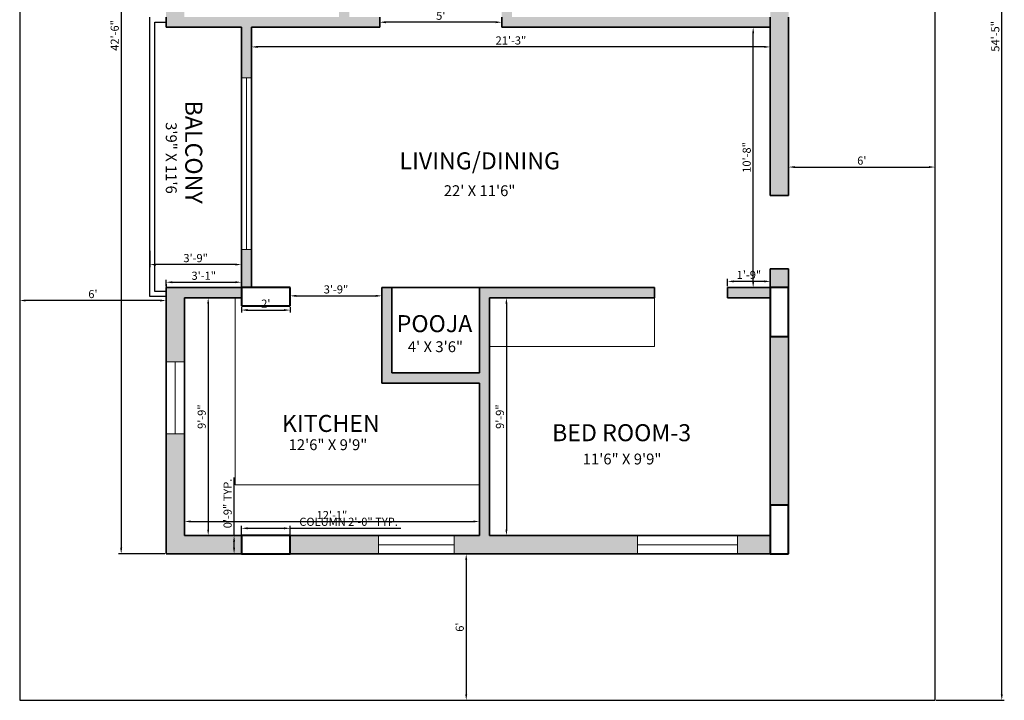
# Model space of a CAD drawing. Units: millimetres. Extents: x 2190 to 2674, y 1487 to 2179.
# Tile 1 of 2: x 2190 to 2674, y 1487 to 1822. Entities that reach past the tile are written whole.
import ezdxf

# ---------------------------------------------------------------- set-up
doc = ezdxf.new("R2010")
doc.units = ezdxf.units.MM
for name, color, linetype, lineweight in [('A-ANNO-DIMS', 2, 'Continuous', 18), ('A-AREA-IDEN', 7, 'Continuous', 18), ('A-WALL', 7, 'Continuous', 35), ('C-PROP', 7, 'Continuous', 25)]:
    doc.layers.add(name, color=color, linetype=linetype, lineweight=lineweight)
for name, color, linetype, lineweight, true_color in [('A-COLS', 240, 'Continuous', 40, 0xed1f24), ('A-FLOR-CASE', 177, 'Continuous', 18, 0x293189), ('A-FLOR-HRAL', 177, 'Continuous', 25, 0x293189), ('A-GLAZ', 177, 'Continuous', 18, 0x293189), ('A-WALL-PATT', 32, 'Continuous', 13, 0xcd6928)]:
    doc.layers.add(name, color=color, linetype=linetype, lineweight=lineweight, true_color=true_color)
doc.styles.get("Standard").update_dxf_attribs({"font": 'arial.ttf'})
doc.dimstyles.new('ISO-25', dxfattribs={"dimtxt": 4, "dimasz": 3, "dimexe": 1.25, "dimexo": 0.625, "dimtad": 1, "dimdec": 0, "dimlunit": 3, "dimtxsty": 'Standard', "dimcen": 2.5, "dimadec": 0, "dimazin": 0, "dimtfac": 1, "dimtdec": 0, "dimtmove": 0, "dimatfit": 3, "dimfxl": 1, "dimarcsym": 0})

# ---------------------------------------------------------------- blocks, each defined once
blk = doc.blocks.new('*D4')
at = {"layer": 'A-ANNO-DIMS', "color": 0, "lineweight": -2, "transparency": 16777216}
for p, q in [((2254.11, 1708.51), (2254.11, 1700.51)), ((2299.11, 1708.51), (2299.11, 1700.51)), ((2296.11, 1701.76), (2257.11, 1701.76))]:
    blk.add_line(p, q, dxfattribs=at)
at = {"layer": 'A-ANNO-DIMS', "color": 0, "transparency": 16777216}
for points in [[(2257.11, 1702.26), (2257.11, 1701.26), (2254.11, 1701.76)], [(2296.11, 1702.26), (2296.11, 1701.26), (2299.11, 1701.76)]]:
    blk.add_solid(points, dxfattribs=at)
at = {"layer": 'Defpoints', "color": 0, "transparency": 16777216}
for p in [(2254.11, 1709.13), (2299.11, 1709.13), (2254.11, 1701.76)]:
    blk.add_point(p, dxfattribs=at)
at = {"layer": 'A-ANNO-DIMS', "color": 0, "transparency": 16777216, "insert": (2276.61, 1704.43), "char_height": 4, "attachment_point": 5}
blk.add_mtext('3\'-9"', dxfattribs=at)
blk = doc.blocks.new('*D5')
at = {"layer": 'A-ANNO-DIMS', "color": 0, "lineweight": -2, "transparency": 16777216}
for p, q in [((2262.11, 1691.07), (2262.11, 1694.32)), ((2299.11, 1691.07), (2299.11, 1694.32)), ((2265.11, 1693.07), (2296.11, 1693.07))]:
    blk.add_line(p, q, dxfattribs=at)
at = {"layer": 'A-ANNO-DIMS', "color": 0, "transparency": 16777216}
for points in [[(2265.11, 1693.57), (2265.11, 1692.57), (2262.11, 1693.07)], [(2296.11, 1693.57), (2296.11, 1692.57), (2299.11, 1693.07)]]:
    blk.add_solid(points, dxfattribs=at)
at = {"layer": 'Defpoints', "color": 0, "transparency": 16777216}
for p in [(2262.11, 1690.45), (2299.11, 1693.07), (2299.11, 1690.45)]:
    blk.add_point(p, dxfattribs=at)
at = {"layer": 'A-ANNO-DIMS', "color": 0, "transparency": 16777216, "insert": (2280.61, 1695.74), "char_height": 4, "attachment_point": 5}
blk.add_mtext('3\'-1"', dxfattribs=at)
blk = doc.blocks.new('*D6')
at = {"layer": 'A-ANNO-DIMS', "color": 0, "lineweight": -2, "transparency": 16777216}
for p, q in [((2299.11, 1680.82), (2299.11, 1678.13)), ((2323.11, 1680.82), (2323.11, 1678.13)), ((2302.11, 1679.38), (2320.11, 1679.38))]:
    blk.add_line(p, q, dxfattribs=at)
at = {"layer": 'A-ANNO-DIMS', "color": 0, "transparency": 16777216}
for points in [[(2302.11, 1679.88), (2302.11, 1678.88), (2299.11, 1679.38)], [(2320.11, 1679.88), (2320.11, 1678.88), (2323.11, 1679.38)]]:
    blk.add_solid(points, dxfattribs=at)
at = {"layer": 'Defpoints', "color": 0, "transparency": 16777216}
for p in [(2299.11, 1681.45), (2323.11, 1681.45), (2323.11, 1679.38)]:
    blk.add_point(p, dxfattribs=at)
at = {"layer": 'A-ANNO-DIMS', "color": 0, "transparency": 16777216, "insert": (2311.11, 1682.02), "char_height": 4, "attachment_point": 5}
blk.add_mtext("2'", dxfattribs=at)
blk = doc.blocks.new('*D7')
at = {"layer": 'A-ANNO-DIMS', "color": 0, "lineweight": -2, "transparency": 16777216}
for p, q in [((2323.11, 1689.82), (2323.11, 1685.11)), ((2368.11, 1689.82), (2368.11, 1685.11)), ((2326.11, 1686.36), (2365.11, 1686.36))]:
    blk.add_line(p, q, dxfattribs=at)
at = {"layer": 'A-ANNO-DIMS', "color": 0, "transparency": 16777216}
for points in [[(2326.11, 1686.86), (2326.11, 1685.86), (2323.11, 1686.36)], [(2365.11, 1686.86), (2365.11, 1685.86), (2368.11, 1686.36)]]:
    blk.add_solid(points, dxfattribs=at)
at = {"layer": 'Defpoints', "color": 0, "transparency": 16777216}
for p in [(2323.11, 1690.45), (2368.11, 1690.45), (2368.11, 1686.36)]:
    blk.add_point(p, dxfattribs=at)
at = {"layer": 'A-ANNO-DIMS', "color": 0, "transparency": 16777216, "insert": (2345.61, 1689.03), "char_height": 4, "attachment_point": 5}
blk.add_mtext('3\'-9"', dxfattribs=at)
blk = doc.blocks.new('*D8')
at = {"layer": 'A-ANNO-DIMS', "color": 0, "lineweight": -2, "transparency": 16777216}
for p, q in [((2271.73, 1685.45), (2284.03, 1685.45)), ((2282.78, 1682.45), (2282.78, 1571.45)), ((2271.73, 1568.45), (2284.03, 1568.45))]:
    blk.add_line(p, q, dxfattribs=at)
at = {"layer": 'A-ANNO-DIMS', "color": 0, "transparency": 16777216}
for points in [[(2282.28, 1682.45), (2283.28, 1682.45), (2282.78, 1685.45)], [(2282.28, 1571.45), (2283.28, 1571.45), (2282.78, 1568.45)]]:
    blk.add_solid(points, dxfattribs=at)
at = {"layer": 'Defpoints', "color": 0, "transparency": 16777216}
for p in [(2271.11, 1685.45), (2271.11, 1568.45), (2282.78, 1568.45)]:
    blk.add_point(p, dxfattribs=at)
at = {"layer": 'A-ANNO-DIMS', "color": 0, "transparency": 16777216, "insert": (2280.11, 1626.95), "char_height": 4, "attachment_point": 5, "rotation": 90}
blk.add_mtext('9\'-9"', dxfattribs=at)
blk = doc.blocks.new('*D9')
at = {"layer": 'A-ANNO-DIMS', "color": 0, "lineweight": -2, "transparency": 16777216}
for p, q in [((2271.11, 1569.07), (2271.11, 1576.65)), ((2274.11, 1575.4), (2413.11, 1575.4)), ((2416.11, 1569.07), (2416.11, 1576.65))]:
    blk.add_line(p, q, dxfattribs=at)
at = {"layer": 'A-ANNO-DIMS', "color": 0, "transparency": 16777216}
for points in [[(2274.11, 1575.9), (2274.11, 1574.9), (2271.11, 1575.4)], [(2413.11, 1575.9), (2413.11, 1574.9), (2416.11, 1575.4)]]:
    blk.add_solid(points, dxfattribs=at)
at = {"layer": 'Defpoints', "color": 0, "transparency": 16777216}
for p in [(2416.11, 1575.4), (2271.11, 1568.45), (2416.11, 1568.45)]:
    blk.add_point(p, dxfattribs=at)
at = {"layer": 'A-ANNO-DIMS', "color": 0, "transparency": 16777216, "insert": (2343.61, 1578.03), "char_height": 4, "attachment_point": 5}
blk.add_mtext('12\'-1"', dxfattribs=at)
blk = doc.blocks.new('*D10')
at = {"layer": 'A-ANNO-DIMS', "color": 0, "lineweight": -2, "transparency": 16777216}
for p, q in [((2421.73, 1685.45), (2430.64, 1685.45)), ((2429.39, 1682.45), (2429.39, 1571.45)), ((2421.73, 1568.45), (2430.64, 1568.45))]:
    blk.add_line(p, q, dxfattribs=at)
at = {"layer": 'A-ANNO-DIMS', "color": 0, "transparency": 16777216}
for points in [[(2428.89, 1682.45), (2429.89, 1682.45), (2429.39, 1685.45)], [(2428.89, 1571.45), (2429.89, 1571.45), (2429.39, 1568.45)]]:
    blk.add_solid(points, dxfattribs=at)
at = {"layer": 'Defpoints', "color": 0, "transparency": 16777216}
for p in [(2421.11, 1685.45), (2421.11, 1568.45), (2429.39, 1568.45)]:
    blk.add_point(p, dxfattribs=at)
at = {"layer": 'A-ANNO-DIMS', "color": 0, "transparency": 16777216, "insert": (2426.72, 1626.95), "char_height": 4, "attachment_point": 5, "rotation": 90}
blk.add_mtext('9\'-9"', dxfattribs=at)
blk = doc.blocks.new('*D11')
at = {"layer": 'A-ANNO-DIMS', "color": 0, "lineweight": -2, "transparency": 16777216}
for p, q in [((2538.11, 1691.07), (2538.11, 1694.73)), ((2559.11, 1691.07), (2559.11, 1694.73)), ((2556.11, 1693.48), (2541.11, 1693.48))]:
    blk.add_line(p, q, dxfattribs=at)
at = {"layer": 'A-ANNO-DIMS', "color": 0, "transparency": 16777216}
for points in [[(2541.11, 1693.98), (2541.11, 1692.98), (2538.11, 1693.48)], [(2556.11, 1693.98), (2556.11, 1692.98), (2559.11, 1693.48)]]:
    blk.add_solid(points, dxfattribs=at)
at = {"layer": 'Defpoints', "color": 0, "transparency": 16777216}
for p in [(2538.11, 1693.48), (2538.11, 1690.45), (2559.11, 1690.45)]:
    blk.add_point(p, dxfattribs=at)
at = {"layer": 'A-ANNO-DIMS', "color": 0, "transparency": 16777216, "insert": (2548.61, 1696.15), "char_height": 4, "attachment_point": 5}
blk.add_mtext('1\'-9"', dxfattribs=at)
blk = doc.blocks.new('*D12')
at = {"layer": 'A-ANNO-DIMS', "color": 0, "lineweight": -2, "transparency": 16777216}
for p, q in [((2558.48, 1818.45), (2549.45, 1818.45)), ((2550.7, 1693.45), (2550.7, 1815.45)), ((2558.48, 1690.45), (2549.45, 1690.45))]:
    blk.add_line(p, q, dxfattribs=at)
at = {"layer": 'A-ANNO-DIMS', "color": 0, "transparency": 16777216}
for points in [[(2550.2, 1815.45), (2551.2, 1815.45), (2550.7, 1818.45)], [(2550.2, 1693.45), (2551.2, 1693.45), (2550.7, 1690.45)]]:
    blk.add_solid(points, dxfattribs=at)
at = {"layer": 'Defpoints', "color": 0, "transparency": 16777216}
for p in [(2550.7, 1818.45), (2559.11, 1818.45), (2559.11, 1690.45)]:
    blk.add_point(p, dxfattribs=at)
at = {"layer": 'A-ANNO-DIMS', "color": 0, "transparency": 16777216, "insert": (2548.03, 1754.45), "char_height": 4, "attachment_point": 5, "rotation": 90}
blk.add_mtext('10\'-8"', dxfattribs=at)
blk = doc.blocks.new('*D13')
at = {"layer": 'A-ANNO-DIMS', "color": 0, "lineweight": -2, "transparency": 16777216}
for p, q in [((2304.11, 1817.82), (2304.11, 1807.55)), ((2559.11, 1817.82), (2559.11, 1807.55)), ((2556.11, 1808.8), (2307.11, 1808.8))]:
    blk.add_line(p, q, dxfattribs=at)
at = {"layer": 'A-ANNO-DIMS', "color": 0, "transparency": 16777216}
for points in [[(2307.11, 1809.3), (2307.11, 1808.3), (2304.11, 1808.8)], [(2556.11, 1809.3), (2556.11, 1808.3), (2559.11, 1808.8)]]:
    blk.add_solid(points, dxfattribs=at)
at = {"layer": 'Defpoints', "color": 0, "transparency": 16777216}
for p in [(2304.11, 1818.45), (2559.11, 1818.45), (2304.11, 1808.8)]:
    blk.add_point(p, dxfattribs=at)
at = {"layer": 'A-ANNO-DIMS', "color": 0, "transparency": 16777216, "insert": (2431.61, 1811.47), "char_height": 4, "attachment_point": 5}
blk.add_mtext('21\'-3"', dxfattribs=at)
blk = doc.blocks.new('*D14')
at = {"layer": 'A-ANNO-DIMS', "color": 0, "lineweight": -2, "transparency": 16777216}
for p, q in [((2367.11, 1819.07), (2367.11, 1822.2)), ((2424.11, 1820.95), (2370.11, 1820.95)), ((2427.11, 1819.07), (2427.11, 1822.2))]:
    blk.add_line(p, q, dxfattribs=at)
at = {"layer": 'A-ANNO-DIMS', "color": 0, "transparency": 16777216}
for points in [[(2370.11, 1821.45), (2370.11, 1820.45), (2367.11, 1820.95)], [(2424.11, 1821.45), (2424.11, 1820.45), (2427.11, 1820.95)]]:
    blk.add_solid(points, dxfattribs=at)
at = {"layer": 'Defpoints', "color": 0, "transparency": 16777216}
for p in [(2367.11, 1820.95), (2367.11, 1818.45), (2427.11, 1818.45)]:
    blk.add_point(p, dxfattribs=at)
at = {"layer": 'A-ANNO-DIMS', "color": 0, "transparency": 16777216, "insert": (2397.11, 1823.61), "char_height": 4, "attachment_point": 5}
blk.add_mtext("5'", dxfattribs=at)
blk = doc.blocks.new('*D21')
at = {"layer": 'A-ANNO-DIMS', "color": 0, "lineweight": -2, "transparency": 16777216}
for p, q in [((2261.48, 2069.45), (2238.76, 2069.45)), ((2240.01, 2066.45), (2240.01, 1562.45)), ((2261.48, 1559.45), (2238.76, 1559.45))]:
    blk.add_line(p, q, dxfattribs=at)
at = {"layer": 'A-ANNO-DIMS', "color": 0, "transparency": 16777216}
for points in [[(2239.51, 2066.45), (2240.51, 2066.45), (2240.01, 2069.45)], [(2239.51, 1562.45), (2240.51, 1562.45), (2240.01, 1559.45)]]:
    blk.add_solid(points, dxfattribs=at)
at = {"layer": 'Defpoints', "color": 0, "transparency": 16777216}
for p in [(2262.11, 2069.45), (2240.01, 1559.45), (2262.11, 1559.45)]:
    blk.add_point(p, dxfattribs=at)
at = {"layer": 'A-ANNO-DIMS', "color": 0, "transparency": 16777216, "insert": (2237.34, 1814.45), "char_height": 4, "attachment_point": 5, "rotation": 90}
blk.add_mtext('42\'-6"', dxfattribs=at)
blk = doc.blocks.new('*D22')
at = {"layer": 'A-ANNO-DIMS', "color": 0, "lineweight": -2, "transparency": 16777216}
for p, q in [((2568.11, 1736.32), (2568.11, 1750.96)), ((2571.11, 1749.71), (2637.11, 1749.71)), ((2640.11, 1736.32), (2640.11, 1750.96))]:
    blk.add_line(p, q, dxfattribs=at)
at = {"layer": 'A-ANNO-DIMS', "color": 0, "transparency": 16777216}
for points in [[(2571.11, 1750.21), (2571.11, 1749.21), (2568.11, 1749.71)], [(2637.11, 1750.21), (2637.11, 1749.21), (2640.11, 1749.71)]]:
    blk.add_solid(points, dxfattribs=at)
at = {"layer": 'Defpoints', "color": 0, "transparency": 16777216}
for p in [(2640.11, 1749.71), (2568.11, 1735.69), (2640.11, 1735.69)]:
    blk.add_point(p, dxfattribs=at)
at = {"layer": 'A-ANNO-DIMS', "color": 0, "transparency": 16777216, "insert": (2604.11, 1752.38), "char_height": 4, "attachment_point": 5}
blk.add_mtext("6'", dxfattribs=at)
blk = doc.blocks.new('*D23')
at = {"layer": 'A-ANNO-DIMS', "color": 0, "lineweight": -2, "transparency": 16777216}
for p, q in [((2404.37, 1559.45), (2410.88, 1559.45)), ((2409.63, 1556.45), (2409.63, 1490.45)), ((2404.37, 1487.45), (2410.88, 1487.45))]:
    blk.add_line(p, q, dxfattribs=at)
at = {"layer": 'A-ANNO-DIMS', "color": 0, "transparency": 16777216}
for points in [[(2409.13, 1556.45), (2410.13, 1556.45), (2409.63, 1559.45)], [(2409.13, 1490.45), (2410.13, 1490.45), (2409.63, 1487.45)]]:
    blk.add_solid(points, dxfattribs=at)
at = {"layer": 'Defpoints', "color": 0, "transparency": 16777216}
for p in [(2403.74, 1559.45), (2403.74, 1487.45), (2409.63, 1487.45)]:
    blk.add_point(p, dxfattribs=at)
at = {"layer": 'A-ANNO-DIMS', "color": 0, "transparency": 16777216, "insert": (2406.96, 1523.45), "char_height": 4, "attachment_point": 5, "rotation": 90}
blk.add_mtext("6'", dxfattribs=at)
blk = doc.blocks.new('*D24')
at = {"layer": 'A-ANNO-DIMS', "color": 0, "lineweight": -2, "transparency": 16777216}
for p, q in [((2190.11, 1692.07), (2190.11, 1682.83)), ((2262.11, 1692.07), (2262.11, 1682.83)), ((2259.11, 1684.08), (2193.11, 1684.08))]:
    blk.add_line(p, q, dxfattribs=at)
at = {"layer": 'A-ANNO-DIMS', "color": 0, "transparency": 16777216}
for points in [[(2193.11, 1684.58), (2193.11, 1683.58), (2190.11, 1684.08)], [(2259.11, 1684.58), (2259.11, 1683.58), (2262.11, 1684.08)]]:
    blk.add_solid(points, dxfattribs=at)
at = {"layer": 'Defpoints', "color": 0, "transparency": 16777216}
for p in [(2190.11, 1692.69), (2262.11, 1692.69), (2190.11, 1684.08)]:
    blk.add_point(p, dxfattribs=at)
at = {"layer": 'A-ANNO-DIMS', "color": 0, "transparency": 16777216, "insert": (2226.11, 1686.74), "char_height": 4, "attachment_point": 5}
blk.add_mtext("6'", dxfattribs=at)
blk = doc.blocks.new('COLUMN-RECT-LONG-Y')
for p, q in [((9, 24), (0, 24)), ((0, 24), (0, 0)), ((9, 0), (9, 24)), ((0, 0), (9, 0))]:
    blk.add_line(p, q)
blk = doc.blocks.new('COLUMN-RECT-LONG-X')
for p, q in [((24, 9), (0, 9)), ((0, 9), (0, 5)), ((0, 5), (0, 0)), ((24, 0), (24, 9)), ((0, 0), (24, 0))]:
    blk.add_line(p, q)
blk = doc.blocks.new('*D30')
at = {"layer": 'A-ANNO-DIMS', "color": 0, "lineweight": -2, "transparency": 16777216}
for p, q in [((2299.11, 1569.07), (2299.11, 1573.3)), ((2323.11, 1569.07), (2323.11, 1573.3)), ((2302.11, 1572.05), (2320.11, 1572.05)), ((2323.11, 1572.05), (2377.46, 1572.05))]:
    blk.add_line(p, q, dxfattribs=at)
at = {"layer": 'A-ANNO-DIMS', "color": 0, "transparency": 16777216}
for points in [[(2302.11, 1572.55), (2302.11, 1571.55), (2299.11, 1572.05)], [(2320.11, 1572.55), (2320.11, 1571.55), (2323.11, 1572.05)]]:
    blk.add_solid(points, dxfattribs=at)
at = {"layer": 'Defpoints', "color": 0, "transparency": 16777216}
for p in [(2299.11, 1568.45), (2323.11, 1572.05), (2323.11, 1568.45)]:
    blk.add_point(p, dxfattribs=at)
at = {"layer": 'A-ANNO-DIMS', "color": 0, "transparency": 16777216, "insert": (2351.79, 1574.74), "char_height": 4, "attachment_point": 5}
blk.add_mtext('COLUMN 2\'-0" TYP.', dxfattribs=at)
blk = doc.blocks.new('*D31')
at = {"layer": 'A-ANNO-DIMS', "color": 0, "lineweight": -2, "transparency": 16777216}
for p, q in [((2295.51, 1568.45), (2295.51, 1597.08)), ((2298.48, 1568.45), (2294.26, 1568.45)), ((2295.51, 1562.45), (2295.51, 1565.45)), ((2298.48, 1559.45), (2294.26, 1559.45))]:
    blk.add_line(p, q, dxfattribs=at)
at = {"layer": 'A-ANNO-DIMS', "color": 0, "transparency": 16777216}
for points in [[(2295.01, 1565.45), (2296.01, 1565.45), (2295.51, 1568.45)], [(2295.01, 1562.45), (2296.01, 1562.45), (2295.51, 1559.45)]]:
    blk.add_solid(points, dxfattribs=at)
at = {"layer": 'Defpoints', "color": 0, "transparency": 16777216}
for p in [(2295.51, 1568.45), (2299.11, 1568.45), (2299.11, 1559.45)]:
    blk.add_point(p, dxfattribs=at)
at = {"layer": 'A-ANNO-DIMS', "color": 0, "transparency": 16777216, "insert": (2292.84, 1584.26), "char_height": 4, "attachment_point": 5, "rotation": 90}
blk.add_mtext('0\'-9" TYP.', dxfattribs=at)
blk = doc.blocks.new('*D33')
at = {"layer": 'A-ANNO-DIMS', "color": 0, "lineweight": -2, "transparency": 16777216}
for p, q in [((2640.73, 2140.55), (2674.16, 2140.55)), ((2672.91, 1490.45), (2672.91, 2137.55)), ((2640.73, 1487.45), (2674.16, 1487.45))]:
    blk.add_line(p, q, dxfattribs=at)
at = {"layer": 'A-ANNO-DIMS', "color": 0, "transparency": 16777216}
for points in [[(2672.41, 2137.55), (2673.41, 2137.55), (2672.91, 2140.55)], [(2672.41, 1490.45), (2673.41, 1490.45), (2672.91, 1487.45)]]:
    blk.add_solid(points, dxfattribs=at)
at = {"layer": 'Defpoints', "color": 0, "transparency": 16777216}
for p in [(2640.11, 2140.55), (2672.91, 2140.55), (2640.11, 1487.45)]:
    blk.add_point(p, dxfattribs=at)
at = {"layer": 'A-ANNO-DIMS', "color": 0, "transparency": 16777216, "insert": (2670.25, 1814), "char_height": 4, "attachment_point": 5, "rotation": 90}
blk.add_mtext('54\'-5"', dxfattribs=at)

msp = doc.modelspace()

# ---------------------------------------------------------------- hatches: boundary and pattern name
at = {"layer": 'A-WALL-PATT'}
h = msp.add_hatch(color=256, dxfattribs=at)
h.dxf.hatch_style = 1
h.paths.add_polyline_path([(2295.11, 2069.45), (2262.11, 2069.45), (2262.11, 2060.45), (2262.11, 1989.95), (2271.11, 1989.95), (2271.11, 2060.45), (2295.11, 2060.45)])
h.paths.add_polyline_path([(2379.55, 2069.45), (2319.11, 2069.45), (2319.11, 2060.45), (2379.55, 2060.45)])
h.paths.add_polyline_path([(2448.39, 2069.45), (2433.11, 2069.45), (2416.52, 2069.45), (2416.52, 2060.45), (2427.11, 2060.45), (2427.11, 1919.45), (2427.11, 1876.45), (2421.86, 1876.45), (2421.86, 1871.45), (2427.11, 1871.45), (2427.11, 1863.71), (2432.11, 1863.71), (2432.11, 1919.45), (2432.11, 1977.45), (2496.64, 1977.45), (2496.64, 1982.45), (2492.11, 1982.45), (2487.11, 1982.45), (2432.11, 1982.45), (2432.11, 2060.45), (2433.11, 2060.45), (2448.39, 2060.45)])
h.paths.add_polyline_path([(2492.11, 2069.45), (2487.11, 2069.45), (2472.59, 2069.45), (2472.59, 2060.45), (2487.11, 2060.45), (2487.11, 2018.45), (2492.11, 2018.45), (2492.11, 2060.45)], flags=17)
h.paths.add_polyline_path([(2568.11, 1823.45), (2568.11, 1865.99), (2559.11, 1865.99), (2559.11, 1823.45), (2559.11, 1735.69), (2568.11, 1735.69)])
h.paths.add_polyline_path([(2559.11, 1823.45), (2432.11, 1823.45), (2432.11, 1826.45), (2427.11, 1826.45), (2427.11, 1823.45), (2427.11, 1818.45), (2559.11, 1818.45)])
h.paths.add_polyline_path([(2568.11, 1982.45), (2568.11, 2044.55), (2559.11, 2044.55), (2559.11, 1982.45), (2551.7, 1982.45), (2551.7, 1977.45), (2559.11, 1977.45), (2559.11, 1889.99), (2568.11, 1889.99)])
h.paths.add_polyline_path([(2352.11, 1871.45), (2384.83, 1871.45), (2384.83, 1876.45), (2364.11, 1876.45), (2364.11, 1919.45), (2355.61, 1919.45), (2355.61, 1914.45), (2359.11, 1914.45), (2359.11, 1876.45), (2320.99, 1876.45), (2320.99, 1871.45), (2347.11, 1871.45), (2347.11, 1859.22), (2352.11, 1859.22)])
h.paths.add_polyline_path([(2297.23, 1876.45), (2271.11, 1876.45), (2271.11, 1883.52), (2262.11, 1883.52), (2262.11, 1871.45), (2262.11, 1854.01), (2271.11, 1854.01), (2271.11, 1871.45), (2297.23, 1871.45)])
h.paths.add_polyline_path([(2367.11, 1823.45), (2352.11, 1823.45), (2352.11, 1828.35), (2347.11, 1828.35), (2347.11, 1823.45), (2271.11, 1823.45), (2271.11, 1830.23), (2262.11, 1830.23), (2262.11, 1823.45), (2262.11, 1818.45), (2271.11, 1818.45), (2299.11, 1818.45), (2299.11, 1793.58), (2304.11, 1793.58), (2304.11, 1818.45), (2367.11, 1818.45)])
h.paths.add_polyline_path([(2271.11, 1929.68), (2262.11, 1929.68), (2262.11, 1919.45), (2262.11, 1907.21), (2271.11, 1907.21), (2271.11, 1914.45), (2324.92, 1914.45), (2324.92, 1919.45), (2271.11, 1919.45)])
h.paths.add_polyline_path([(2299.11, 1690.45), (2271.11, 1690.45), (2262.11, 1690.45), (2262.11, 1685.45), (2262.11, 1653.98), (2271.11, 1653.98), (2271.11, 1685.45), (2296.11, 1685.45), (2299.11, 1685.45), (2299.11, 1686.45)])
h.paths.add_polyline_path([(2304.11, 1709.13), (2299.11, 1709.13), (2299.11, 1690.45), (2304.11, 1690.45)])
h.paths.add_polyline_path([(2299.11, 1568.45), (2271.11, 1568.45), (2271.11, 1592.45), (2271.11, 1593.45), (2271.11, 1618.52), (2262.11, 1618.52), (2262.11, 1568.45), (2262.11, 1559.45), (2271.11, 1559.45), (2299.11, 1559.45), (2299.11, 1564.45)])
h.paths.add_polyline_path([(2366.54, 1568.45), (2323.11, 1568.45), (2323.11, 1559.45), (2366.54, 1559.45)])
h.paths.add_polyline_path([(2493.88, 1568.45), (2421.11, 1568.45), (2421.11, 1593.45), (2421.11, 1685.45), (2502.11, 1685.45), (2502.11, 1690.45), (2421.11, 1690.45), (2416.11, 1690.45), (2416.11, 1685.45), (2416.11, 1648.45), (2373.11, 1648.45), (2373.11, 1690.45), (2368.11, 1690.45), (2368.11, 1648.45), (2368.11, 1643.45), (2373.11, 1643.45), (2416.11, 1643.45), (2416.11, 1568.45), (2403.74, 1568.45), (2403.74, 1559.45), (2421.11, 1559.45), (2493.88, 1559.45)])
h.paths.add_polyline_path([(2559.11, 1568.45), (2543.07, 1568.45), (2543.07, 1559.45), (2559.11, 1559.45)])
h.paths.add_polyline_path([(2568.11, 1666.45), (2559.11, 1666.45), (2559.11, 1583.45), (2568.11, 1583.45)])
h.paths.add_polyline_path([(2559.11, 1690.45), (2538.11, 1690.45), (2538.11, 1685.45), (2559.11, 1685.45)])
h.paths.add_polyline_path([(2568.11, 1699.69), (2559.11, 1699.69), (2559.11, 1690.45), (2568.11, 1690.45)])

# ---------------------------------------------------------------- linework, layer by layer
at = {"layer": 'A-FLOR-CASE'}
for p, q in [((2296.11, 1685.45), (2296.11, 1593.45)), ((2502.11, 1685.45), (2502.11, 1661.45)), ((2502.11, 1661.45), (2421.11, 1661.45)), ((2296.11, 1593.45), (2416.11, 1593.45))]:
    msp.add_line(p, q, dxfattribs=at)
at = {"layer": 'A-FLOR-HRAL'}
for p, q in [((2254.11, 1686.04), (2254.11, 1823.45)), ((2256.61, 1688.54), (2256.61, 1820.95)), ((2256.61, 1820.95), (2262.11, 1820.95)), ((2262.11, 1686.04), (2254.11, 1686.04)), ((2262.11, 1688.54), (2256.61, 1688.54))]:
    msp.add_line(p, q, dxfattribs=at)
at = {"layer": 'A-GLAZ'}
for p, q in [((2301.61, 1793.58), (2301.61, 1709.13)), ((2266.61, 1653.98), (2266.61, 1618.52)), ((2366.54, 1563.95), (2403.74, 1563.95)), ((2493.88, 1563.95), (2543.07, 1563.95))]:
    msp.add_line(p, q, dxfattribs=at)
for points in [[(2299.11, 1793.58), (2304.11, 1793.58), (2304.11, 1709.13), (2299.11, 1709.13)], [(2262.11, 1653.98), (2271.11, 1653.98), (2271.11, 1618.52), (2262.11, 1618.52)], [(2403.74, 1568.45), (2366.54, 1568.45), (2366.54, 1559.45), (2403.74, 1559.45)], [(2543.07, 1568.45), (2493.88, 1568.45), (2493.88, 1559.45), (2543.07, 1559.45)]]:
    msp.add_lwpolyline(points, close=True, dxfattribs=at)
at = {"layer": 'A-WALL'}
for p, q in [((2262.11, 1823.45), (2262.11, 1818.45)), ((2559.11, 1735.69), (2559.11, 1823.45)), ((2568.11, 1735.69), (2568.11, 1823.45)), ((2271.11, 1818.45), (2262.11, 1818.45)), ((2271.11, 1818.45), (2299.11, 1818.45)), ((2271.11, 1818.45), (2299.11, 1818.45)), ((2299.11, 1818.45), (2299.11, 1690.45)), ((2304.11, 1818.45), (2304.11, 1690.45)), ((2304.11, 1818.45), (2367.11, 1818.45)), ((2427.11, 1818.45), (2559.11, 1818.45)), ((2568.11, 1735.69), (2559.11, 1735.69)), ((2559.11, 1690.45), (2559.11, 1699.69)), ((2559.11, 1699.69), (2568.11, 1699.69)), ((2568.11, 1685.45), (2568.11, 1699.69)), ((2271.11, 1690.45), (2262.11, 1690.45)), ((2262.11, 1685.45), (2262.11, 1690.45)), ((2271.11, 1690.45), (2299.11, 1690.45)), ((2368.11, 1648.45), (2368.11, 1690.45)), ((2368.11, 1690.45), (2373.11, 1690.45)), ((2373.11, 1648.45), (2373.11, 1690.45)), ((2373.11, 1690.45), (2416.11, 1690.45)), ((2416.11, 1685.45), (2416.11, 1690.45)), ((2421.11, 1690.45), (2416.11, 1690.45)), ((2502.11, 1690.45), (2421.11, 1690.45)), ((2502.11, 1685.45), (2502.11, 1690.45)), ((2559.11, 1690.45), (2538.11, 1690.45)), ((2559.11, 1690.45), (2538.11, 1690.45)), ((2538.11, 1690.45), (2538.11, 1685.45)), ((2262.11, 1685.45), (2262.11, 1568.45)), ((2271.11, 1685.45), (2299.11, 1685.45)), ((2271.11, 1685.45), (2271.11, 1568.45)), ((2271.11, 1685.45), (2296.11, 1685.45)), ((2416.11, 1648.45), (2416.11, 1685.45)), ((2421.11, 1568.45), (2421.11, 1685.45)), ((2421.11, 1685.45), (2421.11, 1643.45)), ((2502.11, 1685.45), (2421.11, 1685.45)), ((2559.11, 1685.45), (2538.11, 1685.45)), ((2559.11, 1568.45), (2559.11, 1685.45)), ((2568.11, 1568.45), (2568.11, 1685.45)), ((2368.11, 1648.45), (2368.11, 1643.45)), ((2416.11, 1648.45), (2373.11, 1648.45)), ((2373.11, 1643.45), (2368.11, 1643.45)), ((2416.11, 1643.45), (2373.11, 1643.45)), ((2416.11, 1568.45), (2416.11, 1643.45)), ((2271.11, 1592.45), (2271.11, 1593.45)), ((2421.11, 1568.45), (2421.11, 1593.45)), ((2271.11, 1568.45), (2271.11, 1592.45)), ((2262.11, 1568.45), (2262.11, 1559.45)), ((2271.11, 1568.45), (2416.11, 1568.45)), ((2421.11, 1568.45), (2559.11, 1568.45)), ((2568.11, 1568.45), (2568.11, 1559.45)), ((2271.11, 1559.45), (2262.11, 1559.45)), ((2271.11, 1559.45), (2421.11, 1559.45)), ((2421.11, 1559.45), (2559.11, 1559.45)), ((2559.11, 1559.45), (2568.11, 1559.45))]:
    msp.add_line(p, q, dxfattribs=at)
for points in [[(2367.11, 1823.45), (2367.11, 1818.45)], [(2427.11, 1818.45), (2427.11, 1823.45)]]:
    msp.add_lwpolyline(points, dxfattribs=at)
at = {"layer": 'C-PROP'}
for p, q in [((2190.11, 2140.55), (2190.11, 1559.45)), ((2640.11, 1487.45), (2640.11, 2140.55)), ((2190.11, 1559.45), (2190.11, 1487.45)), ((2190.11, 1487.45), (2568.11, 1487.45)), ((2568.11, 1487.45), (2640.11, 1487.45))]:
    msp.add_line(p, q, dxfattribs=at)

# ---------------------------------------------------------------- block references
at = {"layer": 'A-COLS'}
for name, p in [('COLUMN-RECT-LONG-X', (2299.11, 1681.45)), ('COLUMN-RECT-LONG-Y', (2559.11, 1666.45)), ('COLUMN-RECT-LONG-Y', (2559.11, 1559.45)), ('COLUMN-RECT-LONG-X', (2299.11, 1559.45))]:
    msp.add_blockref(name, p, dxfattribs=at)

# ---------------------------------------------------------------- texts
at = {"layer": 'A-AREA-IDEN'}
for s, height, p in [('BALCONY', 8.367, (2271.52, 1782.39)), ('3\'9" X 11\'6', 5.3513, (2261.95, 1771.8))]:
    msp.add_text(s, height=height, rotation=270, dxfattribs=at).set_placement(p)
for s, height, p in [('LIVING/DINING', 8.3669, (2376.79, 1748.6)), ('22\' X 11\'6"', 5.3513, (2398.58, 1735.41)), ('POOJA', 8.367, (2375.44, 1668.52)), ('4\' X 3\'6"', 5.351, (2380.92, 1658.68)), ('KITCHEN', 8.367, (2319.01, 1619.44)), ('BED ROOM-3', 8.367, (2451.82, 1614.88)), ('12\'6" X 9\'9"', 5.3513, (2322.31, 1610.48)), ('11\'6" X 9\'9"', 5.3513, (2466.9, 1603.45))]:
    msp.add_text(s, height=height, dxfattribs=at).set_placement(p)

# ---------------------------------------------------------------- dimensions: what is measured, and where the dimension line sits
at = {"layer": 'A-ANNO-DIMS'}
for base, p1, p2, override, picture, middle in [((2672.91, 2140.55), (2640.11, 1487.45), (2640.11, 2140.55), {"dimdec": 1, "dimlfac": 1, "dimrnd": 0, "dimzin": 1, "dimdsep": 46, "dimlunit": 4, "dimfrac": 2}, '*D33', (2670.25, 1814)), ((2240.01, 1559.45), (2262.11, 2069.45), (2262.11, 1559.45), {"dimclrd": 0, "dimclre": 0, "dimclrt": 0}, '*D21', (2237.34, 1814.45)), ((2550.7, 1818.45), (2559.11, 1690.45), (2559.11, 1818.45), {"dimclrd": 0, "dimclre": 0, "dimclrt": 0}, '*D12', (2548.03, 1754.45)), ((2282.78, 1568.45), (2271.11, 1685.45), (2271.11, 1568.45), {"dimclrd": 0, "dimclre": 0, "dimclrt": 0}, '*D8', (2280.11, 1626.95)), ((2429.39, 1568.45), (2421.11, 1685.45), (2421.11, 1568.45), {"dimclrd": 0, "dimclre": 0, "dimclrt": 0}, '*D10', (2426.72, 1626.95)), ((2409.63, 1487.45), (2403.74, 1559.45), (2403.74, 1487.45), {"dimclrd": 0, "dimclre": 0, "dimclrt": 0}, '*D23', (2406.96, 1523.45))]:
    dim = msp.add_linear_dim(base=base, p1=p1, p2=p2, angle=90, dimstyle='ISO-25', override=override, dxfattribs=at)
    dim.commit()
    dim.dimension.update_dxf_attribs({"geometry": picture, "text_midpoint": middle})
for base, p1, p2, picture, middle in [((2367.11, 1820.95), (2427.11, 1818.45), (2367.11, 1818.45), '*D14', (2397.11, 1823.61)), ((2304.11, 1808.8), (2559.11, 1818.45), (2304.11, 1818.45), '*D13', (2431.61, 1811.47)), ((2640.11, 1749.71), (2568.11, 1735.69), (2640.11, 1735.69), '*D22', (2604.11, 1752.38)), ((2254.11, 1701.76), (2299.11, 1709.13), (2254.11, 1709.13), '*D4', (2276.61, 1704.43)), ((2299.11, 1693.07), (2262.11, 1690.45), (2299.11, 1690.45), '*D5', (2280.61, 1695.74)), ((2538.11, 1693.48), (2559.11, 1690.45), (2538.11, 1690.45), '*D11', (2548.61, 1696.15)), ((2190.11, 1684.08), (2262.11, 1692.69), (2190.11, 1692.69), '*D24', (2226.11, 1686.74)), ((2368.11, 1686.36), (2323.11, 1690.45), (2368.11, 1690.45), '*D7', (2345.61, 1689.03)), ((2323.11, 1679.38), (2299.11, 1681.45), (2323.11, 1681.45), '*D6', (2311.11, 1682.02)), ((2416.11, 1575.4), (2271.11, 1568.45), (2416.11, 1568.45), '*D9', (2343.61, 1578.03))]:
    dim = msp.add_linear_dim(base=base, p1=p1, p2=p2, dimstyle='ISO-25', override={"dimclrd": 0, "dimclre": 0, "dimclrt": 0}, dxfattribs=at)
    dim.commit()
    dim.dimension.update_dxf_attribs({"geometry": picture, "text_midpoint": middle})
dim = msp.add_linear_dim(base=(2295.51, 1568.45), p1=(2299.11, 1559.45), p2=(2299.11, 1568.45), angle=90, text='<> TYP.', dimstyle='ISO-25', override={"dimdec": 1, "dimlfac": 1, "dimrnd": 0, "dimzin": 1, "dimdsep": 46, "dimlunit": 4, "dimfrac": 2}, dxfattribs=at)
dim.commit()
dim.dimension.update_dxf_attribs({"geometry": '*D31', "text_midpoint": (2292.84, 1584.26)})
dim = msp.add_linear_dim(base=(2323.11, 1572.05), p1=(2299.11, 1568.45), p2=(2323.11, 1568.45), text='COLUMN <> TYP.', dimstyle='ISO-25', override={"dimdec": 1, "dimlfac": 1, "dimrnd": 0, "dimzin": 1, "dimdsep": 46, "dimlunit": 4, "dimfrac": 2}, dxfattribs=at)
dim.commit()
dim.dimension.update_dxf_attribs({"geometry": '*D30', "text_midpoint": (2351.79, 1574.74)})

doc.saveas('drawing.dxf')
